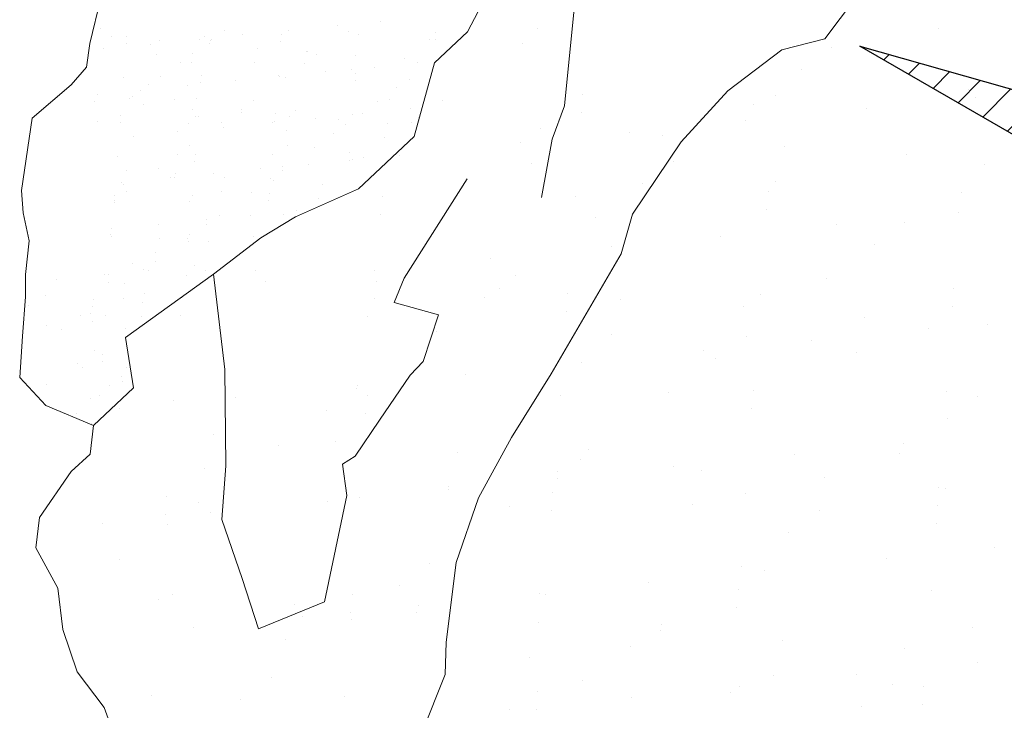
# Model space of a CAD drawing. Units: inches. Extents: x 1986 to 21484, y -1816 to 2016.
# Tile 57 of 85: x 3645.943 to 3651.423, y 1883.641 to 1887.486. Entities that reach past the tile are written whole.
import ezdxf

# ---------------------------------------------------------------- set-up
doc = ezdxf.new("R2010")
doc.units = ezdxf.units.IN
doc.layers.add('L-PLNT', color=84, linetype='Continuous', lineweight=13)
doc.layers.add('vfolhas', color=114, linetype='Continuous', lineweight=5)
doc.layers.add('vfolhas2', color=102, linetype='Continuous')

# ---------------------------------------------------------------- blocks, each defined once
blk = doc.blocks.new('arbusto_PB_verde_grande')
at = {"layer": 'vfolhas'}
h = blk.add_hatch(dxfattribs=at)
h.set_pattern_fill('ANSI31', color=256, scale=0.05, style=0)
h.set_pattern_definition([(45, (-2446.5133113, 50.986076), (-0.004419417382, 0.004419417382), [])])
h.paths.add_polyline_path([(-0.57219, 0.06233), (-0.7153, 0.10298), (-0.67736, 0.08107), (-0.62769, 0.01536), (-0.56347, -0.04095), (-0.26461, -0.0834), (-0.14874, -0.06595), (-0.10151, -0.05877), (-0.20418, -0.0472), (-0.40279, -0.00339)])
h.paths.add_polyline_path([(-0.56347, -0.04095), (-0.58279, -0.02401), (-0.72992, -0.09726), (-0.4334, -0.1679), (-0.41452, -0.15048), (-0.31518, -0.09101), (-0.26461, -0.0834)])
h.paths.add_polyline_path([(-0.2769, -0.47267), (-0.27429, -0.44776), (-0.16328, -0.25376), (0.02625, -0.03934), (-0.21007, -0.20995), (-0.2672, -0.24466), (-0.36485, -0.35697), (-0.42907, -0.46341), (-0.47586, -0.60425), (-0.37946, -0.57603)])
at = {"layer": 'vfolhas2'}
for p, q in [((-0.67736, 0.08107), (-0.7153, 0.10298)), ((-0.7153, 0.10298), (-0.57219, 0.06233))]:
    blk.add_line(p, q, dxfattribs=at)
blk = doc.blocks.new('PLANT-SHRUB')
for p, q in [((2176.9238, 1877.8768), (2176.9238, 1877.8768)), ((2177.3078, 1877.8382), (2177.3078, 1877.8382)), ((2177.2342, 1877.7707), (2177.2342, 1877.7707)), ((2176.8107, 1877.7152), (2176.8107, 1877.7152)), ((2177.3535, 1877.6437), (2177.3535, 1877.6437)), ((2177.5616, 1877.6163), (2177.5616, 1877.6163)), ((2177.1634, 1877.5415), (2177.1634, 1877.5415)), ((2176.4167, 1877.4765), (2176.4167, 1877.4765)), ((2177.4628, 1877.4632), (2177.4628, 1877.4632)), ((2176.8364, 1877.4062), (2176.8364, 1877.4062)), ((2176.5566, 1877.155), (2176.5566, 1877.155)), ((2177.8013, 1877.1527), (2177.8013, 1877.1527)), ((2176.8986, 1877.1067), (2176.8986, 1877.1067)), ((2176.3881, 1877.0476), (2176.3881, 1877.0476)), ((2176.4886, 1877.0876), (2176.4886, 1877.0876)), ((2177.6327, 1877.0453), (2177.6327, 1877.0453)), ((2177.9781, 1877.0678), (2177.9781, 1877.0678)), ((2178.0378, 1877.0554), (2178.0378, 1877.0554)), ((2176.415, 1877.0201), (2176.415, 1877.0201)), ((2175.9092, 1876.799), (2175.9092, 1876.799)), ((2176.1172, 1876.7717), (2176.1172, 1876.7717)), ((2176.4422, 1876.7289), (2176.4422, 1876.7289)), ((2177.6901, 1876.7368), (2177.6901, 1876.7368)), ((2176.3915, 1876.7064), (2176.3915, 1876.7064)), ((2177.4377, 1876.6931), (2177.4377, 1876.6931)), ((2177.6164, 1876.6693), (2177.6164, 1876.6693)), ((2178.4601, 1876.698), (2178.4601, 1876.698)), ((2176.0172, 1876.6556), (2176.0172, 1876.6556)), ((2176.985, 1876.6574), (2176.985, 1876.6574)), ((2177.1931, 1876.63), (2177.1931, 1876.63)), ((2177.518, 1876.5872), (2177.518, 1876.5872)), ((2175.596, 1876.543), (2175.596, 1876.543)), ((2176.8406, 1876.5407), (2176.8406, 1876.5407)), ((2178.0608, 1876.5158), (2178.0608, 1876.5158)), ((2178.0852, 1876.5384), (2178.0852, 1876.5384)), ((2178.2689, 1876.4884), (2178.2689, 1876.4884)), ((2178.5938, 1876.4456), (2178.5938, 1876.4456)), ((2178.8916, 1876.386), (2178.8916, 1876.386)), ((2175.6695, 1876.3369), (2175.6695, 1876.3369)), ((2175.8511, 1876.3317), (2175.8511, 1876.3317)), ((2176.8734, 1876.3366), (2176.8734, 1876.3366)), ((2177.2186, 1876.3048), (2177.2186, 1876.3048)), ((2177.9529, 1876.2977), (2177.9529, 1876.2977)), ((2178.8179, 1876.3185), (2178.8179, 1876.3185)), ((2178.9991, 1876.2844), (2178.9991, 1876.2844)), ((2175.5958, 1876.2694), (2175.5958, 1876.2694)), ((2176.2339, 1876.1542), (2176.2339, 1876.1542)), ((2177.4785, 1876.1519), (2177.4785, 1876.1519)), ((2178.7231, 1876.1496), (2178.7231, 1876.1496)), ((2179.6713, 1876.1487), (2179.1294, 1875.8977)), ((2176.0653, 1876.0468), (2176.0653, 1876.0468)), ((2177.3099, 1876.0445), (2177.3099, 1876.0445)), ((2178.5546, 1876.0423), (2178.5546, 1876.0423)), ((2175.2868, 1875.9752), (2175.2868, 1875.9752)), ((2176.8709, 1875.9862), (2176.8709, 1875.9862)), ((2178.4201, 1875.954), (2178.4201, 1875.954)), ((2175.198, 1875.9049), (2175.198, 1875.9049)), ((2176.3663, 1875.9364), (2176.3663, 1875.9364)), ((2176.7973, 1875.9187), (2176.7973, 1875.9187)), ((2177.4125, 1875.923), (2177.4125, 1875.923)), ((2178.4349, 1875.9279), (2178.4349, 1875.9279)), ((2179.1294, 1875.8977), (2179.0013, 1875.7697)), ((2174.9978, 1875.8842), (2174.9978, 1875.8842)), ((2175.5407, 1875.8127), (2175.5407, 1875.8127)), ((2175.7487, 1875.7854), (2175.7487, 1875.7854)), ((2176.0737, 1875.7426), (2176.0737, 1875.7426)), ((2179.0013, 1875.7697), (2178.6564, 1875.4842)), ((2176.6165, 1875.6711), (2176.6165, 1875.6711)), ((2176.8246, 1875.6437), (2176.8246, 1875.6437)), ((2178.0724, 1875.6354), (2178.0724, 1875.6354)), ((2174.7797, 1875.575), (2174.7797, 1875.575)), ((2174.8503, 1875.5863), (2174.8503, 1875.5863)), ((2176.8483, 1875.5665), (2176.8483, 1875.5665)), ((2177.1495, 1875.6009), (2177.1495, 1875.6009)), ((2177.9987, 1875.5679), (2177.9987, 1875.5679)), ((2179.6216, 1875.6032), (2179.6216, 1875.6032)), ((2174.7766, 1875.5188), (2174.7766, 1875.5188)), ((2175.2732, 1875.5421), (2175.2732, 1875.5421)), ((2175.8259, 1875.5616), (2175.8259, 1875.5616)), ((2176.3995, 1875.5541), (2176.3995, 1875.5541)), ((2176.5178, 1875.5399), (2176.5178, 1875.5399)), ((2177.6924, 1875.5295), (2177.6924, 1875.5295)), ((2177.7624, 1875.5376), (2177.7624, 1875.5376)), ((2177.9277, 1875.5276), (2177.9277, 1875.5276)), ((2178.9739, 1875.5143), (2178.9739, 1875.5143)), ((2179.0071, 1875.5353), (2179.0071, 1875.5353)), ((2177.9004, 1875.5021), (2177.9004, 1875.5021)), ((2178.2253, 1875.4593), (2178.2253, 1875.4593)), ((2178.6564, 1875.4842), (2178.3213, 1875.3069)), ((2178.7682, 1875.3878), (2178.7682, 1875.3878)), ((2178.9762, 1875.3605), (2178.9762, 1875.3605)), ((2178.3213, 1875.3069), (2177.9567, 1875.1888)), ((2179.3011, 1875.3177), (2179.3011, 1875.3177)), ((2176.0518, 1875.2355), (2176.0518, 1875.2355)), ((2179.2739, 1875.2846), (2179.2739, 1875.2846)), ((2179.844, 1875.2462), (2179.844, 1875.2462)), ((2175.2617, 1875.2051), (2175.2617, 1875.2051)), ((2177.9567, 1875.1888), (2177.5527, 1875.0804)), ((2177.6009, 1875.2034), (2177.6009, 1875.2034)), ((2179.2002, 1875.2171), (2179.2002, 1875.2171)), ((2180.052, 1875.2188), (2180.052, 1875.2188)), ((2174.6664, 1875.1556), (2174.6664, 1875.1556)), ((2175.9111, 1875.1533), (2175.9111, 1875.1533)), ((2175.9781, 1875.168), (2175.9781, 1875.168)), ((2176.3411, 1875.1663), (2176.3411, 1875.1663)), ((2177.1557, 1875.1511), (2177.1557, 1875.1511)), ((2177.3873, 1875.1529), (2177.3873, 1875.1529)), ((2178.4003, 1875.1488), (2178.4003, 1875.1488)), ((2178.4097, 1875.1578), (2178.4097, 1875.1578)), ((2179.3424, 1875.1428), (2178.8459, 1874.7963)), ((2179.7128, 1875.001), (2179.3424, 1875.1428)), ((2179.645, 1875.1466), (2179.645, 1875.1466)), ((2177.5527, 1875.0804), (2176.8121, 1874.8603)), ((2179.4892, 1875.1189), (2179.4892, 1875.1189)), ((2175.7425, 1875.046), (2175.7425, 1875.046)), ((2176.9872, 1875.0437), (2176.9872, 1875.0437)), ((2178.2318, 1875.0414), (2178.2318, 1875.0414)), ((2179.4764, 1875.0392), (2179.4764, 1875.0392)), ((2179.5867, 1874.7333), (2179.7128, 1875.001)), ((2176.8121, 1874.8603), (2176.6151, 1874.7421)), ((2177.2532, 1874.8847), (2177.2532, 1874.8847)), ((2178.8024, 1874.8526), (2178.8024, 1874.8526)), ((2180.4016, 1874.8663), (2180.4016, 1874.8663)), ((2180.6967, 1874.8678), (2180.6384, 1874.7317)), ((2175.1722, 1874.8265), (2175.1722, 1874.8265)), ((2175.3802, 1874.7991), (2175.3802, 1874.7991)), ((2175.5803, 1874.8035), (2175.5803, 1874.8035)), ((2176.8231, 1874.7964), (2176.8231, 1874.7964)), ((2177.1795, 1874.8172), (2177.1795, 1874.8172)), ((2178.8459, 1874.7963), (2178.7436, 1874.6519)), ((2178.8459, 1874.7963), (2178.8459, 1874.7963)), ((2175.1665, 1874.7618), (2174.8807, 1874.7126)), ((2175.3833, 1874.6437), (2175.1665, 1874.7618)), ((2175.7052, 1874.7563), (2175.7052, 1874.7563)), ((2175.8007, 1874.7915), (2175.8007, 1874.7915)), ((2176.6151, 1874.7421), (2176.142, 1874.6338)), ((2177.9026, 1874.7575), (2177.9026, 1874.7575)), ((2178.9487, 1874.7442), (2178.9487, 1874.7442)), ((2179.9711, 1874.7491), (2179.9711, 1874.7491)), ((2179.4448, 1874.4183), (2179.5867, 1874.7333)), ((2180.6384, 1874.7317), (2180.6124, 1874.4855)), ((2175.7577, 1874.6043), (2175.3833, 1874.6437)), ((2176.142, 1874.6338), (2175.7577, 1874.6043)), ((2176.248, 1874.6848), (2176.248, 1874.6848)), ((2176.4561, 1874.6574), (2176.4561, 1874.6574)), ((2178.6615, 1874.6683), (2178.4262, 1874.6137)), ((2178.7436, 1874.6519), (2178.6615, 1874.6683)), ((2176.781, 1874.6147), (2176.781, 1874.6147)), ((2178.4262, 1874.6137), (2178.1307, 1874.548)), ((2176.195, 1874.5391), (2176.195, 1874.5391)), ((2177.3239, 1874.5432), (2177.3239, 1874.5432)), ((2177.4397, 1874.5368), (2177.4397, 1874.5368)), ((2178.0267, 1874.5426), (2177.7859, 1874.4113)), ((2178.1307, 1874.548), (2178.0267, 1874.5426)), ((2178.4547, 1874.534), (2178.4547, 1874.534)), ((2178.6843, 1874.5345), (2178.6843, 1874.5345)), ((2179.9289, 1874.5323), (2179.9289, 1874.5323)), ((2177.5319, 1874.5158), (2177.5319, 1874.5158)), ((2177.8568, 1874.473), (2177.8568, 1874.473)), ((2180.0038, 1874.5018), (2180.0038, 1874.5018)), ((2180.6124, 1874.4855), (2180.5087, 1874.2587)), ((2176.7817, 1874.4527), (2176.7817, 1874.4527)), ((2178.381, 1874.4665), (2178.381, 1874.4665)), ((2179.2242, 1874.2136), (2179.4448, 1874.4183)), ((2176.316, 1874.3962), (2176.316, 1874.3962)), ((2177.3621, 1874.3828), (2177.3621, 1874.3828)), ((2177.7859, 1874.4113), (2177.9173, 1874.1926)), ((2178.3845, 1874.3877), (2178.3845, 1874.3877)), ((2178.3997, 1874.4015), (2178.3997, 1874.4015)), ((2178.6077, 1874.3742), (2178.6077, 1874.3742)), ((2176.6545, 1874.1316), (2176.9205, 1874.3286)), ((2176.9205, 1874.3286), (2176.9205, 1874.3286)), ((2178.9326, 1874.3314), (2178.9326, 1874.3314)), ((2179.464, 1874.3488), (2179.464, 1874.3488)), ((2179.4755, 1874.2599), (2179.4755, 1874.2599)), ((2180.5087, 1874.2587), (2180.3725, 1874.0707)), ((2178.8616, 1873.8198), (2179.2242, 1874.2136)), ((2179.6835, 1874.2325), (2179.6835, 1874.2325)), ((2176.8329, 1874.1503), (2176.8329, 1874.1503)), ((2177.9173, 1874.1926), (2177.7859, 1874.1325)), ((2178.0775, 1874.148), (2178.0775, 1874.148)), ((2179.3222, 1874.1457), (2179.3222, 1874.1457)), ((2179.6561, 1874.1832), (2179.6561, 1874.1832)), ((2180.0085, 1874.1897), (2180.0085, 1874.1897)), ((2176.434, 1874.1341), (2176.434, 1874.1341)), ((2176.4771, 1874.043), (2176.6545, 1874.1316)), ((2177.7859, 1874.1325), (2177.1512, 1873.9684)), ((2177.9832, 1874.1019), (2177.9832, 1874.1019)), ((2179.5825, 1874.1157), (2179.5825, 1874.1157)), ((2176.0829, 1873.6984), (2176.4771, 1874.043)), ((2176.3604, 1874.0666), (2176.3604, 1874.0666)), ((2176.6644, 1874.0429), (2176.6644, 1874.0429)), ((2177.909, 1874.0406), (2177.909, 1874.0406)), ((2179.1536, 1874.0384), (2179.1536, 1874.0384)), ((2180.3725, 1874.0707), (2180.3076, 1873.8245)), ((2176.7979, 1874.0263), (2176.7979, 1874.0263)), ((2177.8774, 1873.9874), (2177.8774, 1873.9874)), ((2178.9236, 1873.9741), (2178.9236, 1873.9741)), ((2179.946, 1873.979), (2179.946, 1873.979)), ((2178.5441, 1873.39), (2178.8616, 1873.8198)), ((2180.3076, 1873.8245), (2180.1779, 1873.7143)), ((2180.3076, 1873.8245), (2180.3076, 1873.8245)), ((2177.6355, 1873.7833), (2177.6355, 1873.7833)), ((2177.5618, 1873.7158), (2177.5618, 1873.7158)), ((2179.1847, 1873.7512), (2179.1847, 1873.7512)), ((2180.1779, 1873.7143), (2179.8731, 1873.6495)), ((2179.7304, 1873.6495), (2179.6072, 1873.5458)), ((2179.8731, 1873.6495), (2179.7304, 1873.6495)), ((2176.2908, 1873.6261), (2176.2908, 1873.6261)), ((2176.4125, 1873.6284), (2176.4125, 1873.6284)), ((2177.2044, 1873.5947), (2176.8418, 1873.3742)), ((2177.2044, 1873.5947), (2177.2044, 1873.5947)), ((2177.6299, 1873.5947), (2177.2044, 1873.5947)), ((2177.337, 1873.6127), (2177.337, 1873.6127)), ((2177.9924, 1873.4687), (2177.6299, 1873.5947)), ((2178.3593, 1873.6176), (2178.3593, 1873.6176)), ((2176.9554, 1873.5569), (2176.9554, 1873.5569)), ((2177.1169, 1873.536), (2177.1169, 1873.536)), ((2177.6977, 1873.57), (2177.6977, 1873.57)), ((2179.3007, 1873.5458), (2179.1431, 1873.3112)), ((2179.6072, 1873.5458), (2179.3007, 1873.5458)), ((2179.4388, 1873.5787), (2179.4388, 1873.5787)), ((2179.6072, 1873.5458), (2179.7235, 1873.2843)), ((2177.1634, 1873.5295), (2177.1634, 1873.5295)), ((2177.3309, 1873.4844), (2177.3309, 1873.4844)), ((2177.4883, 1873.4867), (2177.4883, 1873.4867)), ((2177.8288, 1873.4835), (2177.8288, 1873.4835)), ((2178.3615, 1873.5337), (2178.3615, 1873.5337)), ((2179.3223, 1873.4808), (2179.3223, 1873.4808)), ((2179.6061, 1873.5315), (2179.6061, 1873.5315)), ((2177.1132, 1873.4687), (2177.1132, 1873.4687)), ((2177.2635, 1873.4415), (2177.2635, 1873.4415)), ((2177.545, 1873.4531), (2177.545, 1873.4531)), ((2177.5586, 1873.4426), (2177.5586, 1873.4426)), ((2177.7614, 1873.4406), (2177.7614, 1873.4406)), ((2177.9634, 1873.4478), (2177.9634, 1873.4478)), ((2178.2131, 1873.4215), (2177.9924, 1873.4687)), ((2178.837, 1873.4325), (2178.837, 1873.4325)), ((2179.2226, 1873.4288), (2179.2226, 1873.4288)), ((2179.2549, 1873.4379), (2179.2549, 1873.4379)), ((2179.3055, 1873.4544), (2179.3055, 1873.4544)), ((2179.3887, 1873.4435), (2179.3887, 1873.4435)), ((2179.4671, 1873.4493), (2179.4671, 1873.4493)), ((2179.5187, 1873.4264), (2179.5187, 1873.4264)), ((2179.6316, 1873.4308), (2179.6316, 1873.4308)), ((2176.5897, 1873.3742), (2176.3217, 1873.2797)), ((2176.8418, 1873.3742), (2176.5897, 1873.3742)), ((2176.7893, 1873.3718), (2176.7893, 1873.3718)), ((2176.8418, 1873.3742), (2176.8418, 1873.3742)), ((2177.5291, 1873.4156), (2177.5291, 1873.4156)), ((2178.0312, 1873.4153), (2178.0312, 1873.4153)), ((2178.5441, 1873.39), (2178.2131, 1873.4215)), ((2178.2392, 1873.3879), (2178.2392, 1873.3879)), ((2179.1431, 1873.3112), (2178.5441, 1873.39)), ((2177.0065, 1873.3432), (2177.0065, 1873.3432)), ((2177.0897, 1873.3322), (2177.0897, 1873.3322)), ((2177.164, 1873.3513), (2177.164, 1873.3513)), ((2178.5641, 1873.3451), (2178.5641, 1873.3451)), ((2178.7633, 1873.365), (2178.7633, 1873.365)), ((2179.328, 1873.3219), (2179.328, 1873.3219)), ((2176.7503, 1873.2826), (2176.7503, 1873.2826)), ((2176.9103, 1873.3086), (2176.9103, 1873.3086)), ((2177.2197, 1873.3151), (2177.2197, 1873.3151)), ((2177.3288, 1873.3032), (2177.3288, 1873.3032)), ((2177.37, 1873.2698), (2177.37, 1873.2698)), ((2177.4368, 1873.2865), (2177.4368, 1873.2865)), ((2177.52, 1873.2756), (2177.52, 1873.2756)), ((2177.7377, 1873.3052), (2177.7377, 1873.3052)), ((2178.0097, 1873.2753), (2178.0097, 1873.2753)), ((2178.0392, 1873.3023), (2178.0392, 1873.3023)), ((2178.1695, 1873.2896), (2178.1695, 1873.2896)), ((2178.588, 1873.2843), (2178.588, 1873.2843)), ((2178.6588, 1873.2894), (2178.6588, 1873.2894)), ((2178.997, 1873.2863), (2178.997, 1873.2863)), ((2179.107, 1873.2736), (2179.107, 1873.2736)), ((2179.1431, 1873.3112), (2179.1431, 1873.3112)), ((2179.2985, 1873.2949), (2179.2985, 1873.2949)), ((2179.4287, 1873.2707), (2179.4287, 1873.2707)), ((2179.7235, 1873.2843), (2179.7235, 1873.0705)), ((2176.7209, 1873.2556), (2176.7209, 1873.2556)), ((2176.7727, 1873.2562), (2176.7727, 1873.2562)), ((2176.9467, 1873.2396), (2176.9467, 1873.2396)), ((2177.4445, 1873.2387), (2177.4445, 1873.2387)), ((2177.65, 1873.2585), (2177.65, 1873.2585)), ((2177.8522, 1873.2174), (2177.8522, 1873.2174)), ((2177.8671, 1873.2299), (2177.8671, 1873.2299)), ((2177.9424, 1873.2378), (2177.9424, 1873.2378)), ((2177.9504, 1873.2189), (2177.9504, 1873.2189)), ((2178.4402, 1873.2369), (2178.4402, 1873.2369)), ((2178.9381, 1873.236), (2178.9381, 1873.236)), ((2179.315, 1873.2462), (2179.315, 1873.2462)), ((2179.4359, 1873.2351), (2179.4359, 1873.2351)), ((2177.1031, 1873.1606), (2177.1031, 1873.1606)), ((2178.0803, 1873.2018), (2178.0803, 1873.2018)), ((2178.2975, 1873.1732), (2178.2975, 1873.1732)), ((2178.3807, 1873.1623), (2178.3807, 1873.1623)), ((2178.5198, 1873.1619), (2178.5198, 1873.1619)), ((2178.8984, 1873.204), (2178.8984, 1873.204)), ((2179.64, 1873.2035), (2179.64, 1873.2035)), ((2177.2014, 1873.1153), (2177.2014, 1873.1153)), ((2177.2309, 1873.1423), (2177.2309, 1873.1423)), ((2177.5349, 1873.1451), (2177.5349, 1873.1451)), ((2177.7548, 1873.1472), (2177.7548, 1873.1472)), ((2177.8506, 1873.1295), (2177.8506, 1873.1295)), ((2177.9534, 1873.1397), (2177.9534, 1873.1397)), ((2178.3623, 1873.1417), (2178.3623, 1873.1417)), ((2178.4903, 1873.1349), (2178.4903, 1873.1349)), ((2178.5107, 1873.1452), (2178.5107, 1873.1452)), ((2178.7278, 1873.1166), (2178.7278, 1873.1166)), ((2178.7941, 1873.1261), (2178.7941, 1873.1261)), ((2178.811, 1873.1056), (2178.811, 1873.1056)), ((2178.9994, 1873.1449), (2178.9994, 1873.1449)), ((2179.1394, 1873.1491), (2179.1394, 1873.1491)), ((2179.2126, 1873.1208), (2179.2126, 1873.1208)), ((2177.2018, 1873.0841), (2177.2018, 1873.0841)), ((2177.6997, 1873.0832), (2177.6997, 1873.0832)), ((2178.1975, 1873.0823), (2178.1975, 1873.0823)), ((2178.6954, 1873.0814), (2178.6954, 1873.0814)), ((2178.941, 1873.0885), (2178.941, 1873.0885)), ((2179.1581, 1873.0599), (2179.1581, 1873.0599)), ((2179.1932, 1873.0805), (2179.1932, 1873.0805)), ((2179.2413, 1873.049), (2179.2413, 1873.049)), ((2179.7235, 1873.0705), (2179.5549, 1872.9149)), ((2176.9002, 1873.0005), (2176.9002, 1873.0005)), ((2177.1344, 1873.0412), (2177.1344, 1873.0412)), ((2177.3187, 1872.9952), (2177.3187, 1872.9952)), ((2177.5862, 1873.0398), (2177.5862, 1873.0398)), ((2177.6323, 1873.0403), (2177.6323, 1873.0403)), ((2177.7115, 1873.002), (2177.7115, 1873.002)), ((2177.7277, 1872.9971), (2177.7277, 1872.9971)), ((2178.1301, 1873.0394), (2178.1301, 1873.0394)), ((2178.3312, 1872.9891), (2178.3312, 1872.9891)), ((2178.3655, 1873.0005), (2178.3655, 1873.0005)), ((2178.628, 1873.0384), (2178.628, 1873.0384)), ((2178.8309, 1873.0375), (2178.8309, 1873.0375)), ((2178.9709, 1872.9946), (2178.9709, 1872.9946)), ((2179.0003, 1873.0216), (2179.0003, 1873.0216)), ((2179.1258, 1873.0375), (2179.1258, 1873.0375)), ((2179.3713, 1873.0319), (2179.3713, 1873.0319)), ((2177.0423, 1872.9695), (2177.0423, 1872.9695)), ((2177.682, 1872.975), (2177.682, 1872.975)), ((2178.1595, 1872.9816), (2178.1595, 1872.9816)), ((2178.5779, 1872.9763), (2178.5779, 1872.9763)), ((2178.9869, 1872.9782), (2178.9869, 1872.9782)), ((2179.4187, 1872.9627), (2179.4187, 1872.9627)), ((2177.0723, 1872.9206), (2177.0723, 1872.9206)), ((2177.2894, 1872.892), (2177.2894, 1872.892)), ((2177.3726, 1872.8811), (2177.3726, 1872.8811)), ((2179.5549, 1872.9149), (2179.3928, 1872.7659)), ((2177.093, 1872.8526), (2177.093, 1872.8526)), ((2177.3118, 1872.8426), (2177.3118, 1872.8426)), ((2177.3154, 1872.8384), (2177.3154, 1872.8384)), ((2177.5026, 1872.864), (2177.5026, 1872.864)), ((2177.5229, 1872.8292), (2177.5229, 1872.8292)), ((2177.5248, 1872.837), (2177.5248, 1872.837)), ((2177.7197, 1872.8354), (2177.7197, 1872.8354)), ((2177.803, 1872.8244), (2177.803, 1872.8244)), ((2177.8133, 1872.8375), (2177.8133, 1872.8375)), ((2177.9433, 1872.8317), (2177.9433, 1872.8317)), ((2178.1626, 1872.8347), (2178.1626, 1872.8347)), ((2178.1921, 1872.8617), (2178.1921, 1872.8617)), ((2178.3111, 1872.8366), (2178.3111, 1872.8366)), ((2178.3342, 1872.8475), (2178.3342, 1872.8475)), ((2178.3522, 1872.8337), (2178.3522, 1872.8337)), ((2178.809, 1872.8357), (2178.809, 1872.8357)), ((2178.8117, 1872.8488), (2178.8117, 1872.8488)), ((2179.3068, 1872.8348), (2179.3068, 1872.8348)), ((2177.9329, 1872.8073), (2177.9329, 1872.8073)), ((2178.1501, 1872.7787), (2178.1501, 1872.7787)), ((2178.784, 1872.8181), (2178.784, 1872.8181)), ((2179.2025, 1872.8128), (2179.2025, 1872.8128)), ((2179.4136, 1872.8086), (2179.4136, 1872.8086)), ((2178.2333, 1872.7678), (2178.2333, 1872.7678)), ((2178.3633, 1872.7506), (2178.3633, 1872.7506)), ((2178.5804, 1872.7221), (2178.5804, 1872.7221)), ((2178.6727, 1872.7214), (2178.6727, 1872.7214)), ((2179.3928, 1872.7659), (2179.3085, 1872.6752)), ((2177.3086, 1872.6871), (2177.3086, 1872.6871)), ((2177.3544, 1872.6747), (2177.3544, 1872.6747)), ((2177.3838, 1872.7017), (2177.3838, 1872.7017)), ((2177.5706, 1872.6829), (2177.5706, 1872.6829)), ((2177.7176, 1872.6891), (2177.7176, 1872.6891)), ((2178.0035, 1872.6889), (2178.0035, 1872.6889)), ((2178.0178, 1872.6819), (2178.0178, 1872.6819)), ((2178.0684, 1872.682), (2178.0684, 1872.682)), ((2178.1494, 1872.6736), (2178.1494, 1872.6736)), ((2178.5663, 1872.6811), (2178.5663, 1872.6811)), ((2178.5679, 1872.6682), (2178.5679, 1872.6682)), ((2178.6432, 1872.6944), (2178.6432, 1872.6944)), ((2178.6636, 1872.7111), (2178.6636, 1872.7111)), ((2179.3085, 1872.6752), (2179.1658, 1872.552)), ((2177.5031, 1872.6399), (2177.5031, 1872.6399)), ((2177.9441, 1872.6144), (2177.9441, 1872.6144)), ((2178.001, 1872.639), (2178.001, 1872.639)), ((2178.4988, 1872.6381), (2178.4988, 1872.6381)), ((2177.8644, 1872.5614), (2177.8644, 1872.5614)), ((2179.1658, 1872.552), (2179.0815, 1872.416)), ((2177.5147, 1872.529), (2177.5147, 1872.529)), ((2177.8349, 1872.5344), (2177.8349, 1872.5344)), ((2177.9332, 1872.5237), (2177.9332, 1872.5237)), ((2178.0387, 1872.5329), (2178.0387, 1872.5329)), ((2178.3422, 1872.5256), (2178.3422, 1872.5256)), ((2178.4841, 1872.5486), (2178.4841, 1872.5486)), ((2177.5723, 1872.4409), (2177.5723, 1872.4409)), ((2177.827, 1872.4473), (2177.827, 1872.4473)), ((2177.6556, 1872.4299), (2177.6556, 1872.4299)), ((2177.6627, 1872.429), (2177.6627, 1872.429)), ((2177.6758, 1872.3886), (2177.6758, 1872.3886)), ((2177.6841, 1872.4372), (2177.6841, 1872.4372)), ((2177.7855, 1872.4128), (2177.7855, 1872.4128)), ((2177.8707, 1872.4016), (2177.8707, 1872.4016)), ((2178.182, 1872.4363), (2178.182, 1872.4363)), ((2178.3155, 1872.3941), (2178.3155, 1872.3941)), ((2178.345, 1872.4211), (2178.345, 1872.4211)), ((2179.0815, 1872.416), (2179.0037, 1872.3187)), ((2177.7075, 1872.3811), (2177.7075, 1872.3811)), ((2178.0027, 1872.3842), (2178.0027, 1872.3842)), ((2178.0859, 1872.3732), (2178.0859, 1872.3732)), ((2178.1393, 1872.3655), (2178.1393, 1872.3655)), ((2178.1956, 1872.3588), (2178.1956, 1872.3588)), ((2178.2159, 1872.3561), (2178.2159, 1872.3561)), ((2177.9393, 1872.2816), (2177.9393, 1872.2816)), ((2178.433, 1872.3275), (2178.433, 1872.3275)), ((2179.0037, 1872.3187), (2178.6859, 1872.066)), ((2177.8719, 1872.2387), (2177.8719, 1872.2387)), ((2178.1564, 1872.2483), (2178.1564, 1872.2483)), ((2178.3697, 1872.2378), (2178.3697, 1872.2378)), ((2177.9231, 1872.2156), (2177.9231, 1872.2156)), ((2178.3321, 1872.2176), (2178.3321, 1872.2176)), ((2178.0173, 1872.1209), (2178.0173, 1872.1209)), ((2177.9879, 1872.0939), (2177.9879, 1872.0939)), ((2178.1292, 1872.0575), (2178.1292, 1872.0575)), ((2178.2708, 1872.066), (2178.1671, 1871.9818)), ((2178.4005, 1872.079), (2178.2708, 1872.066)), ((2178.4005, 1872.079), (2178.4005, 1872.079)), ((2178.6859, 1872.066), (2178.4005, 1872.079)), ((2178.0529, 1872.0359), (2178.0529, 1872.0359)), ((2178.1671, 1871.9818), (2177.8688, 1871.7874)), ((2178.0685, 1871.9616), (2178.0685, 1871.9616))]:
    blk.add_line(p, q)

msp = doc.modelspace()

# ---------------------------------------------------------------- block references
at = {"layer": 'L-PLNT', "rotation": 223.1883365522388}
msp.add_blockref('PLANT-SHRUB', (3953.27, 4742.9646), dxfattribs=at)
at = {"layer": 'L-PLNT', "xscale": 24.60366729364114, "yscale": 24.60366729364114, "zscale": 24.60366729364114}
msp.add_blockref('arbusto_PB_verde_grande', (3668.2184, 1884.8051), dxfattribs=at)

doc.saveas('drawing.dxf')
